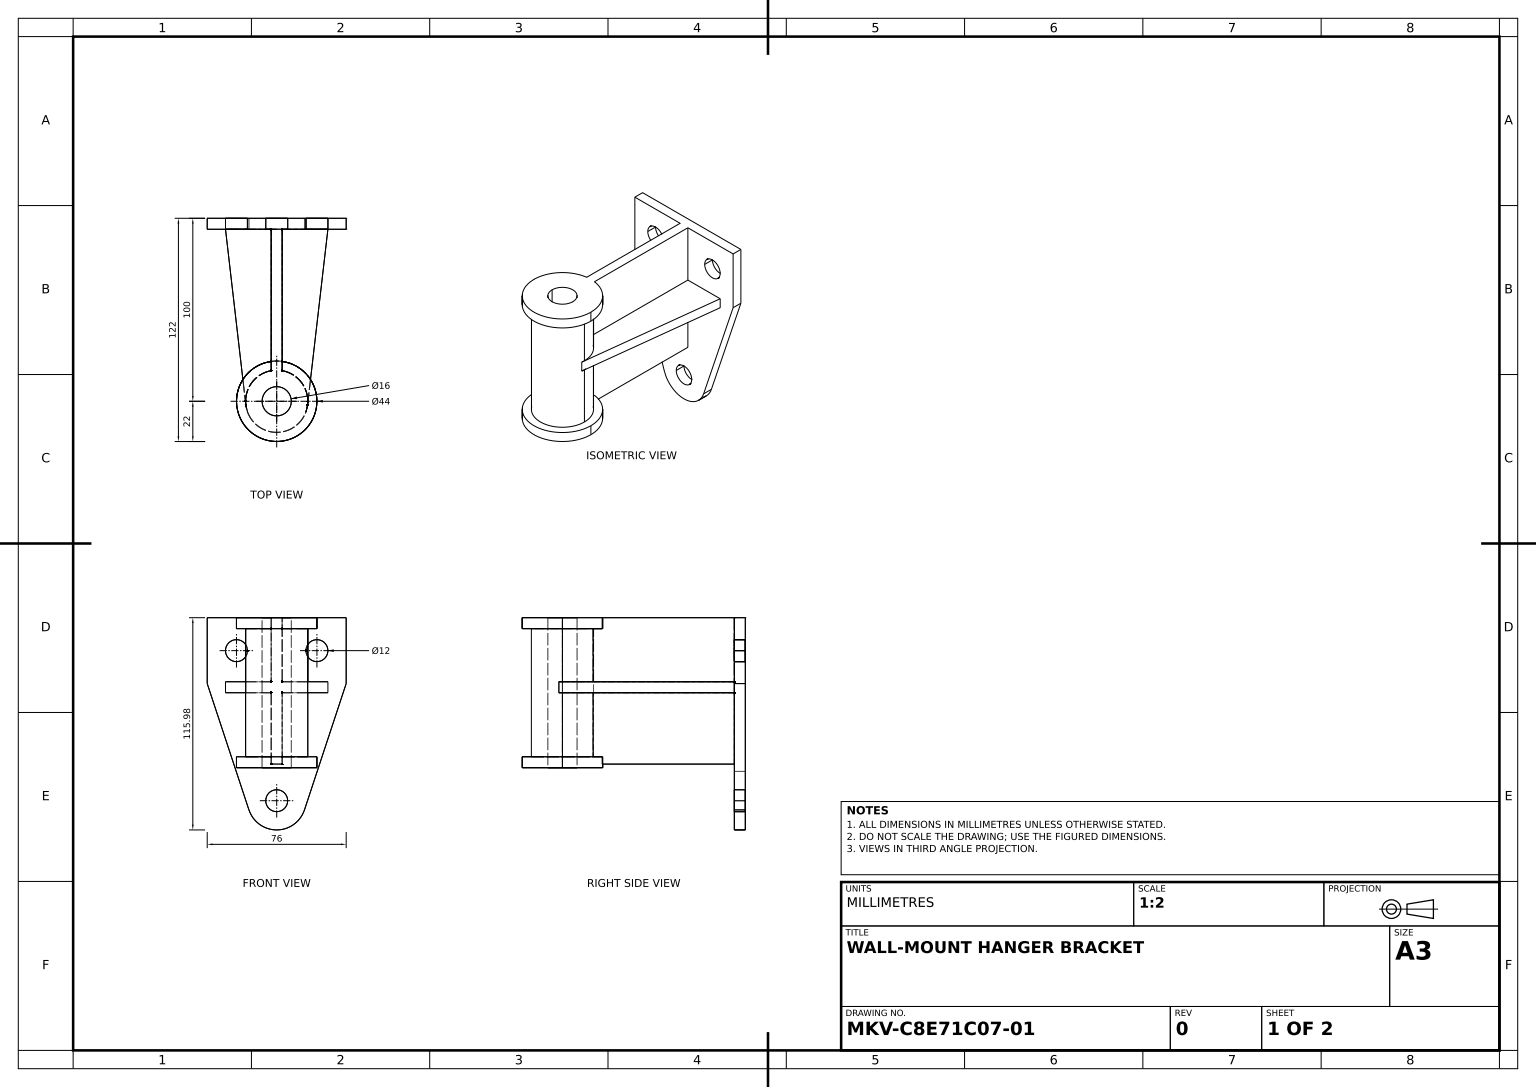
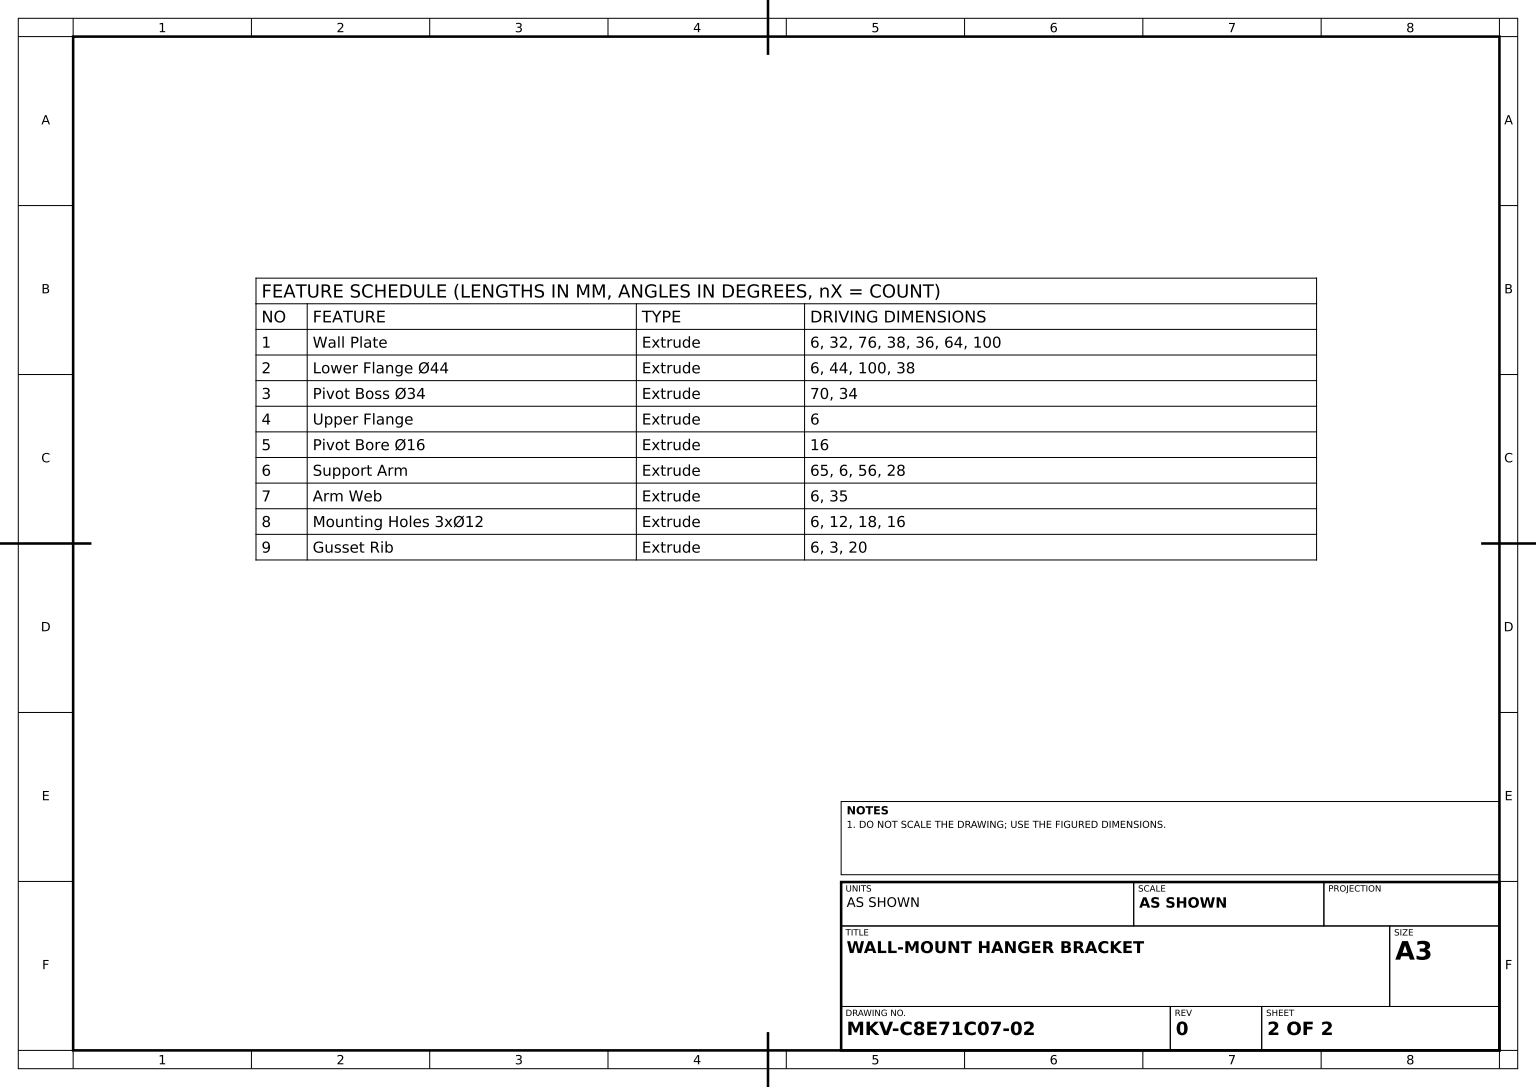
SolidWorks part; units mm, degrees
material "Plain Carbon Steel"
ref_plane "Front Plane" through (0, 0, 0) normal (0, 0, 1) x (1, 0, 0)
ref_plane "Top Plane" through (0, 0, 0) normal (0, 1, 0) x (1, 0, 0)
ref_plane "Right Plane" through (0, 0, 0) normal (1, 0, 0) x (0, 0, -1)
sketch "Wall Plate Sketch" plane through (0, 0, 0) normal (0, 0, 1) x (1, 0, 0)
  line L0 (-38, 64) -> (-15.192, -5.0203)
  line L1 (-38, 100) -> (38, 100)
  line L2 (-38, 100) -> (-38, 64)
  line L4 (38, 100) -> (38, 64)
  line L5 (38, 64) -> (15.192, -5.0203)
  arc A0 (-15.192, -5.0203) -> (15.192, -5.0203) centre (0, 0) ccw
  dimension "D1" = 32
  dimension "D2" = 76
  dimension "D3" = 38
  dimension "D4" = 64
  dimension "D5" = 36
  dimension "D6" = 100
extrude "Wall Plate" add sketch "Wall Plate Sketch" along normal blind 6
sketch "Lower Flange Sketch" plane through (0, 100, 0) normal (0, 1, 0) x (1, 0, 0)
  line L0 (-38, -6) -> (-38, 0) construction
  circle A0 centre (0, -100) radius 22
  dimension "D1" = 44
  dimension "D2" = 100
  dimension "D3" = 38
extrude "Lower Flange Ø44" add sketch "Lower Flange Sketch" against normal blind 6 separate body
sketch "Pivot Boss Sketch" plane through (0, 94, 0) normal (0, -1, 0) x (1, 0, 0)
  circle A0 centre (0, 100) radius 17
  dimension "D1" = 34
extrude "Pivot Boss Ø34" add sketch "Pivot Boss Sketch" along normal blind 70
sketch "Upper Flange Sketch" plane through (0, 24, 0) normal (0, -1, 0) x (1, 0, 0)
  circle A0 centre (0, 100) radius 22 construction
  circle A1 centre (0, 100) radius 22
extrude "Upper Flange" add sketch "Upper Flange Sketch" along normal blind 6
sketch "Pivot Bore Sketch" plane through (0, 100, 0) normal (0, 1, 0) x (1, 0, 0)
  circle A0 centre (0, -100) radius 8
  dimension "D1" = 16
extrude "Pivot Bore Ø16" cut sketch "Pivot Bore Sketch" against normal through all
ref_plane "Support Arm Plane" through (0, 65, 0) normal (0, 1, 0) x (1, 0, 0)
sketch "Support Arm Sketch" plane through (0, 65, 0) normal (0, 1, 0) x (1, 0, 0)
  line L0 (-28, -6) -> (28, -6)
  line L1 (38, -6) -> (-38, -6) construction
  line L2 (-28, -6) -> (-16.8871, -101.9557)
  line L3 (28, -6) -> (16.8871, -101.9557)
  circle A0 centre (0, -100) radius 17 construction
  arc A1 (16.8871, -101.9557) -> (-16.8871, -101.9557) centre (0, -100) ccw
  dimension "D1" = 56
  dimension "D2" = 28
extrude "Support Arm" add sketch "Support Arm Sketch" against normal blind 6
sketch "Arm Web Sketch" plane through (0, 0, 6) normal (0, 0, 1) x (1, 0, 0)
  line L0 (38, 100) -> (-38, 100) construction
  line L1 (-3, 100) -> (3, 100)
  line L2 (-3, 100) -> (-3, 65)
  line L3 (-3, 65) -> (3, 65)
  line L4 (3, 100) -> (3, 65)
  line L5 (28, 65) -> (-28, 65) construction
  line L6 (-38, 100) -> (-38, 64) construction
  dimension "D1" = 6
  dimension "D2" = 35
extrude "Arm Web" add sketch "Arm Web Sketch" along normal up to next
sketch "Mounting Holes Sketch" plane through (0, 0, 6) normal (0, 0, 1) x (1, 0, 0)
  line L0 (-3, 100) -> (-38, 100) construction
  line L1 (38, 100) -> (3, 100) construction
  line L2 (-38, 100) -> (-38, 64) construction
  line L3 (38, 64) -> (38, 100) construction
  circle A0 centre (0, 0) radius 6
  circle A1 centre (-22, 82) radius 6
  circle A2 centre (22, 82) radius 6
  dimension "D1" = 12
  dimension "D2" = 12
  dimension "D3" = 12
  dimension "D4" = 18
  dimension "D5" = 18
  dimension "D6" = 16
  dimension "D7" = 16
extrude "Mounting Holes 3xØ12" cut sketch "Mounting Holes Sketch" against normal blind 6
sketch "Gusset Rib Sketch" plane through (0, 0, 6) normal (0, 0, 1) x (1, 0, 0)
  line L0 (28, 59) -> (-28, 59) construction
  line L1 (-3, 59) -> (3, 59)
  line L2 (-3, 59) -> (-3, 20)
  line L3 (-3, 20) -> (3, 20)
  line L4 (3, 59) -> (3, 20)
  dimension "D1" = 6
  dimension "D2" = 3
  dimension "D3" = 20
extrude "Gusset Rib" add sketch "Gusset Rib Sketch" along normal up to next
